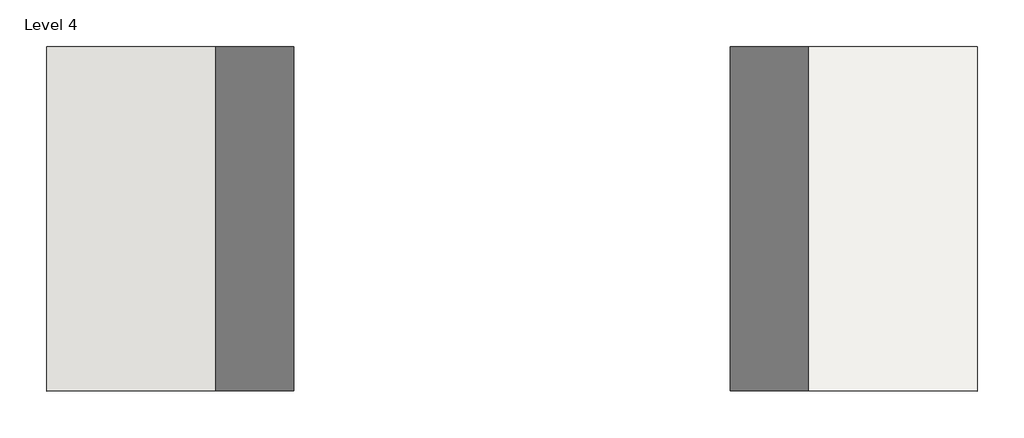
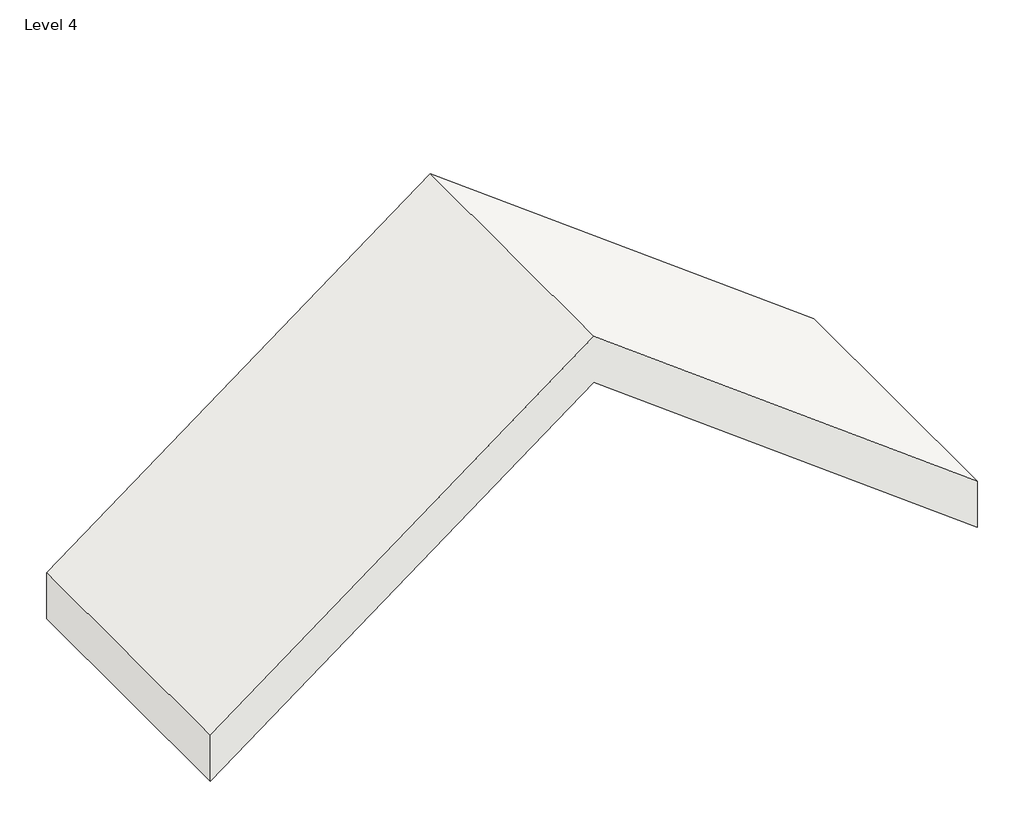
# One storey: 1 roof.
"""IFC4 building model written with IfcOpenShell, lengths in millimetres."""

from ifc_helpers import new_model, si_unit, frame, origin, place, context, project, spatial, polyline, outline, extrude, element, save

model = new_model("IFC4")

# Units and contexts
model_context = context("Model", 3, world=origin())
ifc_project = project(units=[si_unit("LENGTHUNIT", "METRE", prefix="MILLI")], contexts=[model_context])

# Site, building, storey
site = spatial("IfcSite", under=ifc_project)
building = spatial("IfcBuilding", under=site)
storey = spatial("IfcBuildingStorey", under=building, Name="Level 4", Elevation=9144.0)

# Roof
placement = place(None, origin())
element("IfcRoof", 1, ObjectType="Generic - 12\"", at=placement, inside=storey, context=model_context, shape_type="SweptSolid", body=[
    extrude(outline(polyline([(9525.0, -4899.5943664), (11783.8831231, -7911.4385306), (9525.0, -10923.2826947), (9144.0, -10923.2826947), (11402.8831231, -7911.4385306), (9144.0, -4899.5943664), (9525.0, -4899.5943664)])), frame((0.0, -15184.0066876, 0.0), z_axis=(0.0, 1.0, 0.0), x_axis=(0.0, 0.0, 1.0)), (0.0, 0.0, 1.0), 2228.8605387),
])

save(model, "model.ifc")

# Revit data of these elements
# Type "Generic - 12\""
#   Assembly Code = "B1020"
#   Layers, outside or top first: 1' - 0" no material (function 1)
# Element 1 (IfcRoof, "Generic - 12\"")
#   built-in parameter 1001705 = 38.661 (stored number, unit not read)
#   built-in parameter 1001710 = 33615
#   Phase Created = New Construction
#   Materials on its faces: "Default Roof"
# Materials
#   "Default Roof": colour RGB 88 101 114, transparency 0, Cost = 0
